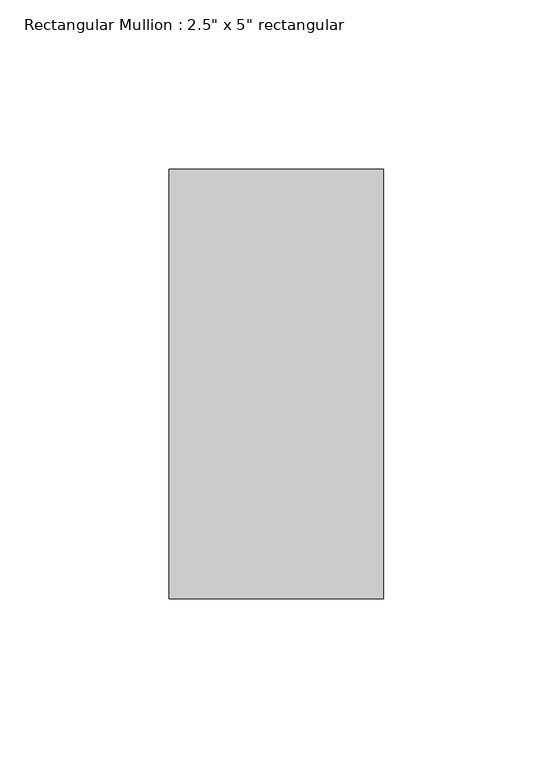
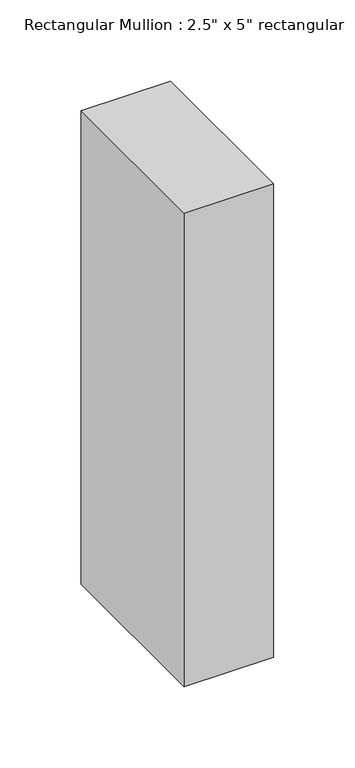
"""IFC4 building model written with IfcOpenShell, lengths in millimetres: member geometry."""

from ifc_helpers import new_model, si_unit, frame, origin, place, context, project, spatial, polyline, outline, extrude, source, transform, mapped, element, save


def member_ffcd2ccf(model_context):
    return source(origin(), model_context, "Body", "SweptSolid", [
        extrude(outline(polyline([(0.0, 63.5), (0.0, -63.5), (-63.5, -63.5), (-63.5, 63.5), (0.0, 63.5)])), frame((0.0, 0.0, -355.6), z_axis=(0.0, 0.0, 1.0), x_axis=(1.0, 0.0, 0.0)), (0.0, 0.0, 1.0), 355.6),
    ])


if __name__ == "__main__":
    model = new_model("IFC4")
    model_context = context("Model", 3, world=origin())
    ifc_project = project(units=[si_unit("LENGTHUNIT", "METRE", prefix="MILLI")], contexts=[model_context])
    site = spatial("IfcSite", under=ifc_project)
    building = spatial("IfcBuilding", under=site)
    placement = place(None, origin())
    member_shape = member_ffcd2ccf(model_context)
    element("IfcMember", 1, ObjectType="Rectangular Mullion : 2.5\" x 5\" rectangular", at=placement, inside=building, context=model_context, shape_type="MappedRepresentation", body=[
        mapped(member_shape, transform((0.0, 0.0, 0.0), x_axis=(1.0, 0.0, 0.0), y_axis=(0.0, 1.0, 0.0), z_axis=(0.0, 0.0, 1.0))),
    ])
    save(model, "model.ifc")

# Revit data of these elements
# Type "Rectangular Mullion : 2.5\" x 5\" rectangular"
#   built-in parameter 1007304 = 0.416667 (stored number, unit not read)
#   built-in parameter 1007301 = 0.104167 (stored number, unit not read)
#   built-in parameter 1007300 = 0.104167 (stored number, unit not read)
